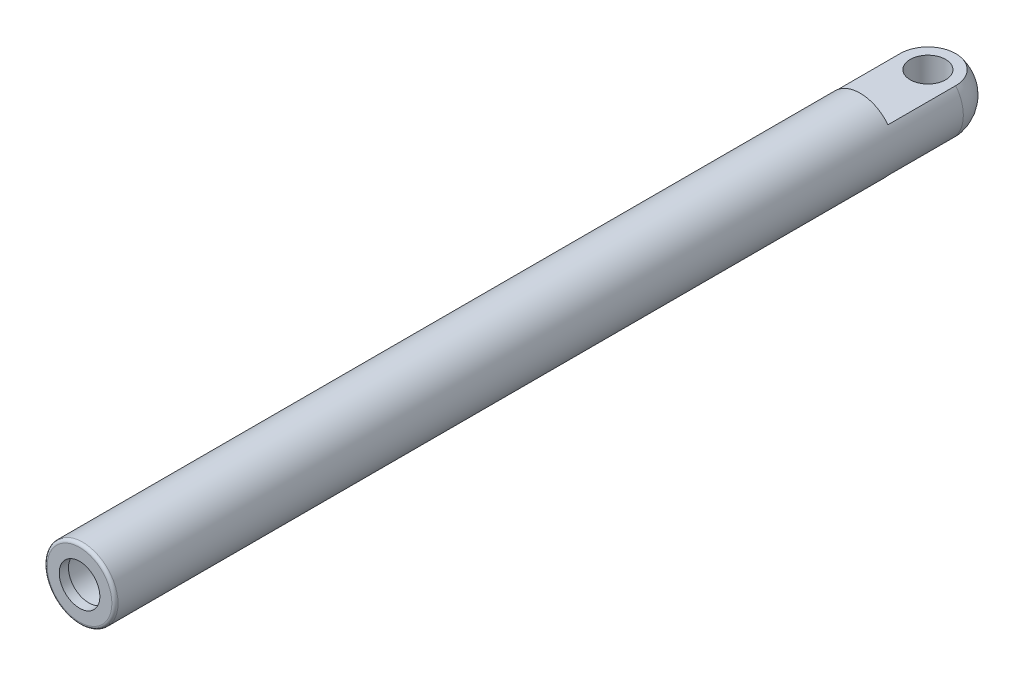
ISO-10303-21;
HEADER;
FILE_DESCRIPTION(('STEP AP214'),'2;1');
FILE_NAME('part.step','',(''),(''),'','','');
FILE_SCHEMA(('AUTOMOTIVE_DESIGN { 1 0 10303 214 1 1 1 1 }'));
ENDSEC;
DATA;
#1=APPLICATION_CONTEXT('core data for automotive mechanical design processes');
#2=APPLICATION_PROTOCOL_DEFINITION('international standard','automotive_design',2000,#1);
#3=PRODUCT_CONTEXT('',#1,'mechanical');
#4=PRODUCT('Part','Part','',(#3));
#5=PRODUCT_RELATED_PRODUCT_CATEGORY('part','',(#4));
#6=PRODUCT_DEFINITION_FORMATION('','',#4);
#7=PRODUCT_DEFINITION_CONTEXT('part definition',#1,'design');
#8=PRODUCT_DEFINITION('design','',#6,#7);
#9=PRODUCT_DEFINITION_SHAPE('','',#8);
#10=(LENGTH_UNIT() NAMED_UNIT(*) SI_UNIT(.MILLI.,.METRE.));
#11=(NAMED_UNIT(*) PLANE_ANGLE_UNIT() SI_UNIT($,.RADIAN.));
#12=(NAMED_UNIT(*) SI_UNIT($,.STERADIAN.) SOLID_ANGLE_UNIT());
#13=UNCERTAINTY_MEASURE_WITH_UNIT(LENGTH_MEASURE(1.E-05),#10,'distance_accuracy_value','');
#14=(GEOMETRIC_REPRESENTATION_CONTEXT(3) GLOBAL_UNCERTAINTY_ASSIGNED_CONTEXT((#13)) GLOBAL_UNIT_ASSIGNED_CONTEXT((#10,
#11,#12)) REPRESENTATION_CONTEXT('',''));
#15=CARTESIAN_POINT('',(0.,0.,0.));
#16=DIRECTION('',(0.,0.,1.));
#17=DIRECTION('',(1.,0.,0.));
#18=AXIS2_PLACEMENT_3D('',#15,#16,#17);
#19=CARTESIAN_POINT('',(0.,0.,1450.));
#20=DIRECTION('',(0.,0.,-1.));
#21=DIRECTION('',(-1.,0.,0.));
#22=AXIS2_PLACEMENT_3D('',#19,#20,#21);
#23=CYLINDRICAL_SURFACE('',#22,115.);
#24=CARTESIAN_POINT('',(0.,0.,1440.));
#25=DIRECTION('',(0.,0.,1.));
#26=DIRECTION('',(1.,0.,0.));
#27=AXIS2_PLACEMENT_3D('',#24,#25,#26);
#28=CIRCLE('',#27,115.);
#29=CARTESIAN_POINT('',(115.,0.,1440.));
#30=VERTEX_POINT('',#29);
#31=EDGE_CURVE('E11',#30,#30,#28,.F.);
#32=ORIENTED_EDGE('',*,*,#31,.T.);
#33=EDGE_LOOP('',(#32));
#34=FACE_BOUND('',#33,.T.);
#35=DIRECTION('',(0.,0.,-1.));
#36=VECTOR('',#35,1.);
#37=CARTESIAN_POINT('',(-90.2686961244041,71.2499999999999,1450.));
#38=LINE('',#37,#36);
#39=CARTESIAN_POINT('',(-90.2686961244041,71.2499999999999,-1085.));
#40=VERTEX_POINT('',#39);
#41=CARTESIAN_POINT('',(-90.2686961244041,71.2499999999999,-1305.));
#42=VERTEX_POINT('',#41);
#43=EDGE_CURVE('E96',#40,#42,#38,.T.);
#44=ORIENTED_EDGE('',*,*,#43,.T.);
#45=CARTESIAN_POINT('',(0.,0.,-1305.));
#46=DIRECTION('',(0.,0.,1.));
#47=DIRECTION('',(1.,0.,0.));
#48=AXIS2_PLACEMENT_3D('',#45,#46,#47);
#49=CIRCLE('',#48,115.);
#50=CARTESIAN_POINT('',(-90.2686961244041,-71.2499999999999,-1305.));
#51=VERTEX_POINT('',#50);
#52=EDGE_CURVE('E53',#42,#51,#49,.T.);
#53=ORIENTED_EDGE('',*,*,#52,.T.);
#54=DIRECTION('',(0.,0.,-1.));
#55=VECTOR('',#54,1.);
#56=CARTESIAN_POINT('',(-90.2686961244041,-71.2499999999999,1450.));
#57=LINE('',#56,#55);
#58=CARTESIAN_POINT('',(-90.2686961244041,-71.2499999999999,-1085.));
#59=VERTEX_POINT('',#58);
#60=EDGE_CURVE('E107',#51,#59,#57,.F.);
#61=ORIENTED_EDGE('',*,*,#60,.T.);
#62=CARTESIAN_POINT('',(0.,0.,-1085.));
#63=DIRECTION('',(0.,0.,1.));
#64=DIRECTION('',(1.,0.,0.));
#65=AXIS2_PLACEMENT_3D('',#62,#63,#64);
#66=CIRCLE('',#65,115.);
#67=CARTESIAN_POINT('',(90.2686961244041,-71.2499999999999,-1085.));
#68=VERTEX_POINT('',#67);
#69=EDGE_CURVE('E97',#59,#68,#66,.T.);
#70=ORIENTED_EDGE('',*,*,#69,.T.);
#71=DIRECTION('',(0.,0.,-1.));
#72=VECTOR('',#71,1.);
#73=CARTESIAN_POINT('',(90.2686961244041,-71.2499999999999,1450.));
#74=LINE('',#73,#72);
#75=CARTESIAN_POINT('',(90.2686961244041,-71.2499999999999,-1305.));
#76=VERTEX_POINT('',#75);
#77=EDGE_CURVE('E90',#68,#76,#74,.T.);
#78=ORIENTED_EDGE('',*,*,#77,.T.);
#79=CARTESIAN_POINT('',(90.2686961244041,71.2499999999999,-1305.));
#80=VERTEX_POINT('',#79);
#81=EDGE_CURVE('E84',#76,#80,#49,.T.);
#82=ORIENTED_EDGE('',*,*,#81,.T.);
#83=DIRECTION('',(0.,0.,-1.));
#84=VECTOR('',#83,1.);
#85=CARTESIAN_POINT('',(90.2686961244041,71.2499999999999,1450.));
#86=LINE('',#85,#84);
#87=CARTESIAN_POINT('',(90.2686961244041,71.2499999999999,-1085.));
#88=VERTEX_POINT('',#87);
#89=EDGE_CURVE('E64',#80,#88,#86,.F.);
#90=ORIENTED_EDGE('',*,*,#89,.T.);
#91=CARTESIAN_POINT('',(0.,0.,-1085.));
#92=DIRECTION('',(0.,0.,1.));
#93=DIRECTION('',(1.,0.,0.));
#94=AXIS2_PLACEMENT_3D('',#91,#92,#93);
#95=CIRCLE('',#94,115.);
#96=EDGE_CURVE('E82',#88,#40,#95,.T.);
#97=ORIENTED_EDGE('',*,*,#96,.T.);
#98=EDGE_LOOP('',(#44,#53,#61,#70,#78,#82,#90,#97));
#99=FACE_BOUND('',#98,.T.);
#100=ADVANCED_FACE('F39',(#34,#99),#23,.T.);
#101=CARTESIAN_POINT('',(0.,0.,1450.));
#102=DIRECTION('',(0.,0.,1.));
#103=DIRECTION('',(1.,0.,0.));
#104=AXIS2_PLACEMENT_3D('',#101,#102,#103);
#105=PLANE('',#104);
#106=CARTESIAN_POINT('',(0.,0.,1450.));
#107=DIRECTION('',(0.,0.,1.));
#108=DIRECTION('',(1.,0.,0.));
#109=AXIS2_PLACEMENT_3D('',#106,#107,#108);
#110=CIRCLE('',#109,105.);
#111=CARTESIAN_POINT('',(105.,0.,1450.));
#112=VERTEX_POINT('',#111);
#113=EDGE_CURVE('E50',#112,#112,#110,.T.);
#114=ORIENTED_EDGE('',*,*,#113,.T.);
#115=EDGE_LOOP('',(#114));
#116=FACE_BOUND('',#115,.T.);
#117=CARTESIAN_POINT('',(0.,0.,1450.));
#118=DIRECTION('',(0.,0.,1.));
#119=DIRECTION('',(1.,0.,0.));
#120=AXIS2_PLACEMENT_3D('',#117,#118,#119);
#121=CIRCLE('',#120,66.);
#122=CARTESIAN_POINT('',(66.,0.,1450.));
#123=VERTEX_POINT('',#122);
#124=EDGE_CURVE('E171',#123,#123,#121,.T.);
#125=ORIENTED_EDGE('',*,*,#124,.F.);
#126=EDGE_LOOP('',(#125));
#127=FACE_BOUND('',#126,.T.);
#128=ADVANCED_FACE('F111',(#116,#127),#105,.T.);
#129=CARTESIAN_POINT('',(-1450.,-252.083782696414,-1085.));
#130=DIRECTION('',(0.,0.,1.));
#131=DIRECTION('',(1.,0.,0.));
#132=AXIS2_PLACEMENT_3D('',#129,#130,#131);
#133=PLANE('',#132);
#134=DIRECTION('',(1.,0.,0.));
#135=VECTOR('',#134,1.);
#136=CARTESIAN_POINT('',(-1450.,-71.2499999999999,-1085.));
#137=LINE('',#136,#135);
#138=EDGE_CURVE('E184',#59,#68,#137,.T.);
#139=ORIENTED_EDGE('',*,*,#138,.T.);
#140=ORIENTED_EDGE('',*,*,#69,.F.);
#141=EDGE_LOOP('',(#139,#140));
#142=FACE_BOUND('',#141,.T.);
#143=ADVANCED_FACE('F134',(#142),#133,.F.);
#144=CARTESIAN_POINT('',(-1450.,-71.2499999999999,-1085.));
#145=DIRECTION('',(0.,1.,0.));
#146=DIRECTION('',(0.,0.,1.));
#147=AXIS2_PLACEMENT_3D('',#144,#145,#146);
#148=PLANE('',#147);
#149=CARTESIAN_POINT('',(0.,-71.2499999999998,-1305.));
#150=DIRECTION('',(0.,1.,0.));
#151=DIRECTION('',(0.,0.,1.));
#152=AXIS2_PLACEMENT_3D('',#149,#150,#151);
#153=CIRCLE('',#152,57.5);
#154=CARTESIAN_POINT('',(0.,-71.2499999999998,-1247.5));
#155=VERTEX_POINT('',#154);
#156=EDGE_CURVE('E106',#155,#155,#153,.F.);
#157=ORIENTED_EDGE('',*,*,#156,.F.);
#158=EDGE_LOOP('',(#157));
#159=FACE_BOUND('',#158,.T.);
#160=ORIENTED_EDGE('',*,*,#60,.F.);
#161=CARTESIAN_POINT('',(0.,-71.2499999999999,-1305.));
#162=DIRECTION('',(0.,1.,0.));
#163=DIRECTION('',(0.,0.,1.));
#164=AXIS2_PLACEMENT_3D('',#161,#162,#163);
#165=CIRCLE('',#164,90.2686961244041);
#166=EDGE_CURVE('E185',#51,#76,#165,.F.);
#167=ORIENTED_EDGE('',*,*,#166,.T.);
#168=ORIENTED_EDGE('',*,*,#77,.F.);
#169=ORIENTED_EDGE('',*,*,#138,.F.);
#170=EDGE_LOOP('',(#160,#167,#168,#169));
#171=FACE_BOUND('',#170,.T.);
#172=ADVANCED_FACE('F138',(#159,#171),#148,.F.);
#173=CARTESIAN_POINT('',(-1450.,252.083782696414,-1085.));
#174=DIRECTION('',(0.,0.,1.));
#175=DIRECTION('',(1.,0.,0.));
#176=AXIS2_PLACEMENT_3D('',#173,#174,#175);
#177=PLANE('',#176);
#178=DIRECTION('',(1.,0.,0.));
#179=VECTOR('',#178,1.);
#180=CARTESIAN_POINT('',(-1450.,71.2499999999999,-1085.));
#181=LINE('',#180,#179);
#182=EDGE_CURVE('E92',#40,#88,#181,.T.);
#183=ORIENTED_EDGE('',*,*,#182,.F.);
#184=ORIENTED_EDGE('',*,*,#96,.F.);
#185=EDGE_LOOP('',(#183,#184));
#186=FACE_BOUND('',#185,.T.);
#187=ADVANCED_FACE('F142',(#186),#177,.F.);
#188=CARTESIAN_POINT('',(-1450.,71.2499999999999,-1085.));
#189=DIRECTION('',(0.,-1.,0.));
#190=DIRECTION('',(0.,0.,-1.));
#191=AXIS2_PLACEMENT_3D('',#188,#189,#190);
#192=PLANE('',#191);
#193=CARTESIAN_POINT('',(0.,71.2499999999998,-1305.));
#194=DIRECTION('',(0.,-1.,0.));
#195=DIRECTION('',(0.,0.,-1.));
#196=AXIS2_PLACEMENT_3D('',#193,#194,#195);
#197=CIRCLE('',#196,57.5);
#198=CARTESIAN_POINT('',(0.,71.2499999999998,-1362.5));
#199=VERTEX_POINT('',#198);
#200=EDGE_CURVE('E100',#199,#199,#197,.F.);
#201=ORIENTED_EDGE('',*,*,#200,.F.);
#202=EDGE_LOOP('',(#201));
#203=FACE_BOUND('',#202,.T.);
#204=ORIENTED_EDGE('',*,*,#89,.F.);
#205=CARTESIAN_POINT('',(0.,71.2499999999999,-1305.));
#206=DIRECTION('',(0.,-1.,0.));
#207=DIRECTION('',(0.,0.,-1.));
#208=AXIS2_PLACEMENT_3D('',#205,#206,#207);
#209=CIRCLE('',#208,90.2686961244041);
#210=EDGE_CURVE('E76',#80,#42,#209,.F.);
#211=ORIENTED_EDGE('',*,*,#210,.T.);
#212=ORIENTED_EDGE('',*,*,#43,.F.);
#213=ORIENTED_EDGE('',*,*,#182,.T.);
#214=EDGE_LOOP('',(#204,#211,#212,#213));
#215=FACE_BOUND('',#214,.T.);
#216=ADVANCED_FACE('F91',(#203,#215),#192,.F.);
#217=CARTESIAN_POINT('',(0.,-1450.,-1305.));
#218=DIRECTION('',(0.,1.,0.));
#219=DIRECTION('',(0.,0.,1.));
#220=AXIS2_PLACEMENT_3D('',#217,#218,#219);
#221=CYLINDRICAL_SURFACE('',#220,57.5);
#222=ORIENTED_EDGE('',*,*,#200,.T.);
#223=EDGE_LOOP('',(#222));
#224=FACE_BOUND('',#223,.T.);
#225=ORIENTED_EDGE('',*,*,#156,.T.);
#226=EDGE_LOOP('',(#225));
#227=FACE_BOUND('',#226,.T.);
#228=ADVANCED_FACE('F133',(#224,#227),#221,.F.);
#229=CARTESIAN_POINT('',(0.,0.,-1305.));
#230=DIRECTION('',(0.,0.,1.));
#231=DIRECTION('',(1.,0.,0.));
#232=AXIS2_PLACEMENT_3D('',#229,#230,#231);
#233=SPHERICAL_SURFACE('',#232,115.);
#234=ORIENTED_EDGE('',*,*,#52,.F.);
#235=ORIENTED_EDGE('',*,*,#210,.F.);
#236=ORIENTED_EDGE('',*,*,#81,.F.);
#237=ORIENTED_EDGE('',*,*,#166,.F.);
#238=EDGE_LOOP('',(#234,#235,#236,#237));
#239=FACE_BOUND('',#238,.T.);
#240=ADVANCED_FACE('F78',(#239),#233,.T.);
#241=CARTESIAN_POINT('',(81.,0.,-1035.));
#242=DIRECTION('',(0.,0.,-1.));
#243=DIRECTION('',(-1.,0.,0.));
#244=AXIS2_PLACEMENT_3D('',#241,#242,#243);
#245=PLANE('',#244);
#246=CARTESIAN_POINT('',(0.,0.,-1035.));
#247=DIRECTION('',(0.,0.,1.));
#248=DIRECTION('',(1.,0.,0.));
#249=AXIS2_PLACEMENT_3D('',#246,#247,#248);
#250=CIRCLE('',#249,81.);
#251=CARTESIAN_POINT('',(81.,0.,-1035.));
#252=VERTEX_POINT('',#251);
#253=EDGE_CURVE('E89',#252,#252,#250,.T.);
#254=ORIENTED_EDGE('',*,*,#253,.T.);
#255=EDGE_LOOP('',(#254));
#256=FACE_BOUND('',#255,.T.);
#257=ADVANCED_FACE('F154',(#256),#245,.F.);
#258=CARTESIAN_POINT('',(0.,0.,1450.));
#259=DIRECTION('',(0.,0.,1.));
#260=DIRECTION('',(1.,0.,0.));
#261=AXIS2_PLACEMENT_3D('',#258,#259,#260);
#262=CYLINDRICAL_SURFACE('',#261,81.);
#263=ORIENTED_EDGE('',*,*,#253,.F.);
#264=EDGE_LOOP('',(#263));
#265=FACE_BOUND('',#264,.T.);
#266=CARTESIAN_POINT('',(0.,0.,1420.));
#267=DIRECTION('',(0.,0.,1.));
#268=DIRECTION('',(1.,0.,0.));
#269=AXIS2_PLACEMENT_3D('',#266,#267,#268);
#270=CIRCLE('',#269,81.);
#271=CARTESIAN_POINT('',(81.,0.,1420.));
#272=VERTEX_POINT('',#271);
#273=EDGE_CURVE('E168',#272,#272,#270,.T.);
#274=ORIENTED_EDGE('',*,*,#273,.T.);
#275=EDGE_LOOP('',(#274));
#276=FACE_BOUND('',#275,.T.);
#277=ADVANCED_FACE('F158',(#265,#276),#262,.F.);
#278=CARTESIAN_POINT('',(66.,0.,1420.));
#279=DIRECTION('',(0.,0.,1.));
#280=DIRECTION('',(1.,0.,0.));
#281=AXIS2_PLACEMENT_3D('',#278,#279,#280);
#282=PLANE('',#281);
#283=ORIENTED_EDGE('',*,*,#273,.F.);
#284=EDGE_LOOP('',(#283));
#285=FACE_BOUND('',#284,.T.);
#286=CARTESIAN_POINT('',(0.,0.,1420.));
#287=DIRECTION('',(0.,0.,1.));
#288=DIRECTION('',(1.,0.,0.));
#289=AXIS2_PLACEMENT_3D('',#286,#287,#288);
#290=CIRCLE('',#289,66.);
#291=CARTESIAN_POINT('',(66.,0.,1420.));
#292=VERTEX_POINT('',#291);
#293=EDGE_CURVE('E175',#292,#292,#290,.T.);
#294=ORIENTED_EDGE('',*,*,#293,.T.);
#295=EDGE_LOOP('',(#294));
#296=FACE_BOUND('',#295,.T.);
#297=ADVANCED_FACE('F123',(#285,#296),#282,.F.);
#298=CARTESIAN_POINT('',(0.,0.,1450.));
#299=DIRECTION('',(0.,0.,1.));
#300=DIRECTION('',(1.,0.,0.));
#301=AXIS2_PLACEMENT_3D('',#298,#299,#300);
#302=CYLINDRICAL_SURFACE('',#301,66.);
#303=ORIENTED_EDGE('',*,*,#293,.F.);
#304=EDGE_LOOP('',(#303));
#305=FACE_BOUND('',#304,.T.);
#306=ORIENTED_EDGE('',*,*,#124,.T.);
#307=EDGE_LOOP('',(#306));
#308=FACE_BOUND('',#307,.T.);
#309=ADVANCED_FACE('F120',(#305,#308),#302,.F.);
#310=CARTESIAN_POINT('',(0.,0.,1440.));
#311=DIRECTION('',(0.,0.,1.));
#312=DIRECTION('',(1.,0.,0.));
#313=AXIS2_PLACEMENT_3D('',#310,#311,#312);
#314=TOROIDAL_SURFACE('',#313,105.,10.);
#315=ORIENTED_EDGE('',*,*,#31,.F.);
#316=EDGE_LOOP('',(#315));
#317=FACE_BOUND('',#316,.T.);
#318=ORIENTED_EDGE('',*,*,#113,.F.);
#319=EDGE_LOOP('',(#318));
#320=FACE_BOUND('',#319,.T.);
#321=ADVANCED_FACE('F41',(#317,#320),#314,.T.);
#322=CLOSED_SHELL('',(#100,#128,#143,#172,#187,#216,#228,#240,#257,#277,#297,#309,#321));
#323=MANIFOLD_SOLID_BREP('B2',#322);
#324=ADVANCED_BREP_SHAPE_REPRESENTATION('',(#18,#323),#14);
#325=SHAPE_DEFINITION_REPRESENTATION(#9,#324);
ENDSEC;
END-ISO-10303-21;
